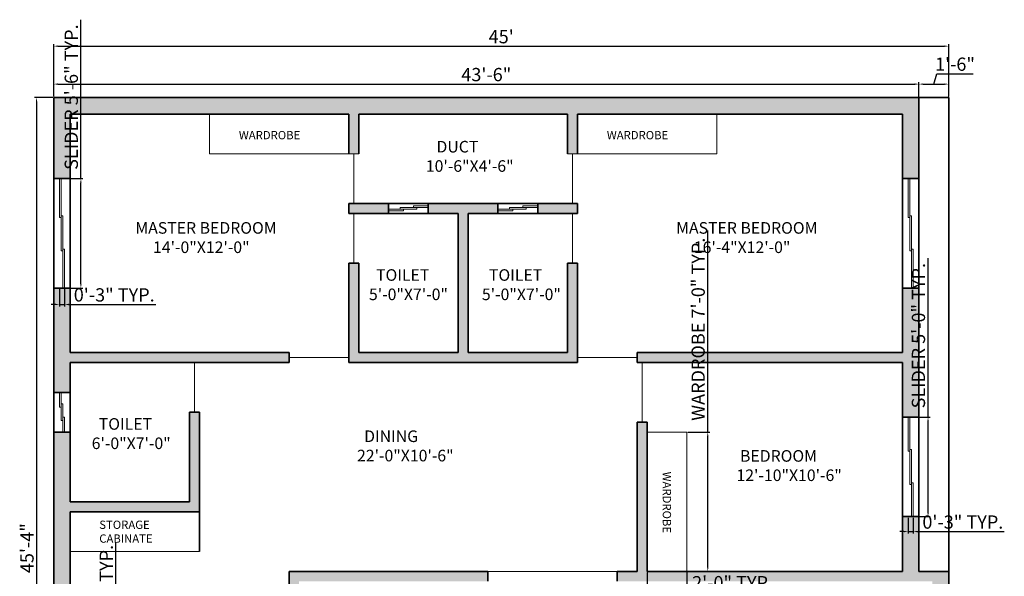
# Model space of a CAD drawing. Units: inches. Extents: x 3491 to 6898, y 1360 to 2019.
# Tile 5 of 9: x 4140 to 4734, y 1683 to 2019. Entities that reach past the tile are written whole.
import ezdxf

# ---------------------------------------------------------------- set-up
doc = ezdxf.new("R2010")
doc.units = ezdxf.units.IN
for name, color, linetype, lineweight in [('A-ANNO-DIMS', 2, 'Continuous', 18), ('A-ANNO-TEXT', 7, 'Continuous', 18), ('A-AREA-IDEN', 7, 'Continuous', 18), ('A-DOOR', 4, 'Continuous', 18), ('A-FLOR-CASE', 8, 'Continuous', 18), ('A-GLAZ', 5, 'Continuous', 18), ('A-WALL', 7, 'Continuous', 35), ('A-WALL-PATT', 8, 'Continuous', 13)]:
    doc.layers.add(name, color=color, linetype=linetype, lineweight=lineweight)
doc.layers.add('A-WALL-OPEN', color=251, linetype='Continuous', lineweight=13, true_color=0x636466)
doc.styles.get("Standard").update_dxf_attribs({"font": 'arial.ttf'})
doc.dimstyles.new('ISO-25', dxfattribs={"dimtxt": 8, "dimasz": 2.5, "dimexe": 1.25, "dimexo": 0.625, "dimtad": 1, "dimdec": 1, "dimlunit": 3, "dimtxsty": 'Standard', "dimcen": 2.5, "dimclrt": 1, "dimadec": 0, "dimazin": 0, "dimtfac": 1, "dimtdec": 1, "dimtmove": 0, "dimatfit": 3, "dimfxl": 1, "dimarcsym": 0})

# ---------------------------------------------------------------- blocks, each defined once
blk = doc.blocks.new('*D15')
at = {"layer": 'A-ANNO-DIMS', "color": 0, "lineweight": -2, "transparency": 16777216}
for p, q in [((4160.3, 1972.99), (4160.3, 1981.69)), ((4162.8, 1980.44), (4679.8, 1980.44)), ((4682.3, 1972.99), (4682.3, 1981.69))]:
    blk.add_line(p, q, dxfattribs=at)
at = {"layer": 'A-ANNO-DIMS', "color": 0, "transparency": 16777216}
for points in [[(4162.8, 1980.85), (4162.8, 1980.02), (4160.3, 1980.44)], [(4679.8, 1980.85), (4679.8, 1980.02), (4682.3, 1980.44)]]:
    blk.add_solid(points, dxfattribs=at)
at = {"layer": 'Defpoints', "color": 0, "transparency": 16777216}
for p in [(4682.3, 1980.44), (4160.3, 1972.37), (4682.3, 1972.37)]:
    blk.add_point(p, dxfattribs=at)
at = {"layer": 'A-ANNO-DIMS', "color": 0, "transparency": 16777216, "insert": (4421.3, 1985.15), "char_height": 8, "attachment_point": 5}
blk.add_mtext('43\'-6"', dxfattribs=at)
blk = doc.blocks.new('*D16')
at = {"layer": 'A-ANNO-DIMS', "color": 0, "lineweight": -2, "transparency": 16777216}
for p, q in [((4691.3, 1980.44), (4693.19, 1986.71)), ((4693.19, 1986.71), (4714.95, 1986.71)), ((4682.3, 1972.99), (4682.3, 1981.69)), ((4684.8, 1980.44), (4697.8, 1980.44)), ((4700.3, 1972.99), (4700.3, 1981.69))]:
    blk.add_line(p, q, dxfattribs=at)
at = {"layer": 'A-ANNO-DIMS', "color": 0, "transparency": 16777216}
for points in [[(4684.8, 1980.85), (4684.8, 1980.02), (4682.3, 1980.44)], [(4697.8, 1980.85), (4697.8, 1980.02), (4700.3, 1980.44)]]:
    blk.add_solid(points, dxfattribs=at)
at = {"layer": 'Defpoints', "color": 0, "transparency": 16777216}
for p in [(4700.3, 1980.44), (4682.3, 1972.37), (4700.3, 1972.37)]:
    blk.add_point(p, dxfattribs=at)
at = {"layer": 'A-ANNO-DIMS', "color": 0, "transparency": 16777216, "insert": (4704.07, 1991.42), "char_height": 8, "attachment_point": 5}
blk.add_mtext('1\'-6"', dxfattribs=at)
blk = doc.blocks.new('*D13')
at = {"layer": 'A-ANNO-DIMS', "color": 0, "lineweight": -2, "transparency": 16777216}
for p, q in [((4160.3, 1972.99), (4160.3, 2004.59)), ((4162.8, 2003.34), (4697.8, 2003.34)), ((4700.3, 1972.99), (4700.3, 2004.59))]:
    blk.add_line(p, q, dxfattribs=at)
at = {"layer": 'A-ANNO-DIMS', "color": 0, "transparency": 16777216}
for points in [[(4162.8, 2003.76), (4162.8, 2002.92), (4160.3, 2003.34)], [(4697.8, 2003.76), (4697.8, 2002.92), (4700.3, 2003.34)]]:
    blk.add_solid(points, dxfattribs=at)
at = {"layer": 'Defpoints', "color": 0, "transparency": 16777216}
for p in [(4700.3, 2003.34), (4160.3, 1972.37), (4700.3, 1972.37)]:
    blk.add_point(p, dxfattribs=at)
at = {"layer": 'A-ANNO-DIMS', "color": 0, "transparency": 16777216, "insert": (4430.3, 2008.03), "char_height": 8, "attachment_point": 5}
blk.add_mtext("45'", dxfattribs=at)
blk = doc.blocks.new('*D17')
at = {"layer": 'A-ANNO-DIMS', "color": 0, "lineweight": -2, "transparency": 16777216}
for p, q in [((4159.68, 1972.37), (4148.67, 1972.37)), ((4149.92, 1969.87), (4149.92, 1430.87)), ((4159.68, 1428.37), (4148.67, 1428.37))]:
    blk.add_line(p, q, dxfattribs=at)
at = {"layer": 'A-ANNO-DIMS', "color": 0, "transparency": 16777216}
for points in [[(4149.51, 1969.87), (4150.34, 1969.87), (4149.92, 1972.37)], [(4149.51, 1430.87), (4150.34, 1430.87), (4149.92, 1428.37)]]:
    blk.add_solid(points, dxfattribs=at)
at = {"layer": 'Defpoints', "color": 0, "transparency": 16777216}
for p in [(4160.3, 1972.37), (4149.92, 1428.37), (4160.3, 1428.37)]:
    blk.add_point(p, dxfattribs=at)
at = {"layer": 'A-ANNO-DIMS', "color": 0, "transparency": 16777216, "insert": (4145.23, 1700.37), "char_height": 8, "attachment_point": 5, "rotation": 90}
blk.add_mtext('45\'-4"', dxfattribs=at)
blk = doc.blocks.new('WIN-SLIDER-24IN')
for p, q in [((0, 1), (17, 1)), ((0, 0), (9, 0)), ((7, 1), (7, 2)), ((7, 2), (24, 2)), ((9, 0), (9, 1)), ((15, 2), (15, 3)), ((15, 3), (24, 3)), ((17, 1), (17, 2))]:
    blk.add_line(p, q)
blk = doc.blocks.new('WIN-SLIDER-66IN')
for p, q in [((0, 42.5), (0, 66)), ((1, 22.5), (1, 66)), ((1, 42.5), (0, 42.5)), ((2, 43.5), (1, 43.5)), ((2, 0), (2, 43.5)), ((2, 22.5), (1, 22.5)), ((3, 23.5), (2, 23.5)), ((3, 0), (3, 23.5))]:
    blk.add_line(p, q)
blk = doc.blocks.new('WIN-SLIDER-60IN')
for p, q in [((0, 39.5), (0, 60)), ((1, 19.5), (1, 60)), ((1, 39.5), (0, 39.5)), ((2, 40.5), (1, 40.5)), ((2, 0), (2, 40.5)), ((2, 19.5), (1, 19.5)), ((3, 20.5), (2, 20.5)), ((3, 0), (3, 20.5))]:
    blk.add_line(p, q)
blk = doc.blocks.new('WARDROBE-84X24')
for q in [(0, 84), (24, 0)]:
    blk.add_line((24, 84), q)
blk = doc.blocks.new('*D114')
at = {"layer": 'A-ANNO-DIMS', "color": 0, "lineweight": -2, "transparency": 16777216}
for p, q in [((4176.7, 1923.37), (4176.7, 2019.32)), ((4167.43, 1923.37), (4177.95, 1923.37)), ((4176.7, 1859.87), (4176.7, 1920.87)), ((4167.43, 1857.37), (4177.95, 1857.37))]:
    blk.add_line(p, q, dxfattribs=at)
at = {"layer": 'A-ANNO-DIMS', "color": 0, "transparency": 16777216}
for points in [[(4176.29, 1920.87), (4177.12, 1920.87), (4176.7, 1923.37)], [(4176.29, 1859.87), (4177.12, 1859.87), (4176.7, 1857.37)]]:
    blk.add_solid(points, dxfattribs=at)
at = {"layer": 'Defpoints', "color": 0, "transparency": 16777216}
for p in [(4166.8, 1923.37), (4176.7, 1923.37), (4166.8, 1857.37)]:
    blk.add_point(p, dxfattribs=at)
at = {"layer": 'A-ANNO-DIMS', "color": 1, "transparency": 16777216, "insert": (4171.94, 1972.59), "char_height": 8, "attachment_point": 5, "rotation": 90}
blk.add_mtext('SLIDER 5\'-6" TYP.', dxfattribs=at)
blk = doc.blocks.new('*D115')
at = {"layer": 'A-ANNO-DIMS', "color": 0, "lineweight": -2, "transparency": 16777216}
for p, q in [((4163.8, 1856.74), (4163.8, 1846.22)), ((4166.8, 1856.74), (4166.8, 1846.22)), ((4161.3, 1847.47), (4158.8, 1847.47)), ((4163.8, 1847.47), (4166.8, 1847.47)), ((4169.3, 1847.47), (4221.82, 1847.47))]:
    blk.add_line(p, q, dxfattribs=at)
at = {"layer": 'A-ANNO-DIMS', "color": 0, "transparency": 16777216}
for points in [[(4161.3, 1847.88), (4161.3, 1847.05), (4163.8, 1847.47)], [(4169.3, 1847.88), (4169.3, 1847.05), (4166.8, 1847.47)]]:
    blk.add_solid(points, dxfattribs=at)
at = {"layer": 'Defpoints', "color": 0, "transparency": 16777216}
for p in [(4163.8, 1857.37), (4166.8, 1857.37), (4166.8, 1847.47)]:
    blk.add_point(p, dxfattribs=at)
at = {"layer": 'A-ANNO-DIMS', "color": 1, "transparency": 16777216, "insert": (4196.81, 1852.18), "char_height": 8, "attachment_point": 5}
blk.add_mtext('0\'-3" TYP.', dxfattribs=at)
blk = doc.blocks.new('*D118')
at = {"layer": 'A-ANNO-DIMS', "color": 0, "lineweight": -2, "transparency": 16777216}
for p, q in [((4687.8, 1779.37), (4687.8, 1875.32)), ((4679.43, 1779.37), (4689.05, 1779.37)), ((4687.8, 1721.87), (4687.8, 1776.87)), ((4679.43, 1719.37), (4689.05, 1719.37))]:
    blk.add_line(p, q, dxfattribs=at)
at = {"layer": 'A-ANNO-DIMS', "color": 0, "transparency": 16777216}
for points in [[(4687.39, 1776.87), (4688.22, 1776.87), (4687.8, 1779.37)], [(4687.39, 1721.87), (4688.22, 1721.87), (4687.8, 1719.37)]]:
    blk.add_solid(points, dxfattribs=at)
at = {"layer": 'Defpoints', "color": 0, "transparency": 16777216}
for p in [(4678.8, 1779.37), (4687.8, 1779.37), (4678.8, 1719.37)]:
    blk.add_point(p, dxfattribs=at)
at = {"layer": 'A-ANNO-DIMS', "color": 1, "transparency": 16777216, "insert": (4683.04, 1828.59), "char_height": 8, "attachment_point": 5, "rotation": 90}
blk.add_mtext('SLIDER 5\'-0" TYP.', dxfattribs=at)
blk = doc.blocks.new('*D119')
at = {"layer": 'A-ANNO-DIMS', "color": 0, "lineweight": -2, "transparency": 16777216}
for p, q in [((4675.8, 1718.74), (4675.8, 1709.12)), ((4678.8, 1718.74), (4678.8, 1709.12)), ((4673.3, 1710.37), (4670.8, 1710.37)), ((4675.8, 1710.37), (4678.8, 1710.37)), ((4681.3, 1710.37), (4733.82, 1710.37))]:
    blk.add_line(p, q, dxfattribs=at)
at = {"layer": 'A-ANNO-DIMS', "color": 0, "transparency": 16777216}
for points in [[(4673.3, 1710.78), (4673.3, 1709.95), (4675.8, 1710.37)], [(4681.3, 1710.78), (4681.3, 1709.95), (4678.8, 1710.37)]]:
    blk.add_solid(points, dxfattribs=at)
at = {"layer": 'Defpoints', "color": 0, "transparency": 16777216}
for p in [(4675.8, 1719.37), (4678.8, 1719.37), (4678.8, 1710.37)]:
    blk.add_point(p, dxfattribs=at)
at = {"layer": 'A-ANNO-DIMS', "color": 1, "transparency": 16777216, "insert": (4708.81, 1715.08), "char_height": 8, "attachment_point": 5}
blk.add_mtext('0\'-3" TYP.', dxfattribs=at)
blk = doc.blocks.new('*D122')
at = {"layer": 'A-ANNO-DIMS', "color": 0, "lineweight": -2, "transparency": 16777216}
for p, q in [((4554.9, 1770.37), (4554.9, 1892.13)), ((4542.93, 1770.37), (4556.15, 1770.37)), ((4554.9, 1688.87), (4554.9, 1767.87)), ((4542.93, 1686.37), (4556.15, 1686.37))]:
    blk.add_line(p, q, dxfattribs=at)
at = {"layer": 'A-ANNO-DIMS', "color": 0, "transparency": 16777216}
for points in [[(4554.49, 1767.87), (4555.32, 1767.87), (4554.9, 1770.37)], [(4554.49, 1688.87), (4555.32, 1688.87), (4554.9, 1686.37)]]:
    blk.add_solid(points, dxfattribs=at)
at = {"layer": 'Defpoints', "color": 0, "transparency": 16777216}
for p in [(4542.3, 1770.37), (4554.9, 1770.37), (4542.3, 1686.37)]:
    blk.add_point(p, dxfattribs=at)
at = {"layer": 'A-ANNO-DIMS', "color": 1, "transparency": 16777216, "insert": (4550.14, 1832.5), "char_height": 8, "attachment_point": 5, "rotation": 90}
blk.add_mtext('WARDROBE 7\'-0" TYP.', dxfattribs=at)
blk = doc.blocks.new('*D123')
at = {"layer": 'A-ANNO-DIMS', "color": 0, "lineweight": -2, "transparency": 16777216}
for p, q in [((4518.3, 1685.74), (4518.3, 1672.52)), ((4542.3, 1685.74), (4542.3, 1672.52)), ((4520.8, 1673.77), (4539.8, 1673.77)), ((4542.3, 1673.77), (4594.96, 1673.77))]:
    blk.add_line(p, q, dxfattribs=at)
at = {"layer": 'A-ANNO-DIMS', "color": 0, "transparency": 16777216}
for points in [[(4520.8, 1674.18), (4520.8, 1673.35), (4518.3, 1673.77)], [(4539.8, 1674.18), (4539.8, 1673.35), (4542.3, 1673.77)]]:
    blk.add_solid(points, dxfattribs=at)
at = {"layer": 'Defpoints', "color": 0, "transparency": 16777216}
for p in [(4518.3, 1686.37), (4542.3, 1686.37), (4542.3, 1673.77)]:
    blk.add_point(p, dxfattribs=at)
at = {"layer": 'A-ANNO-DIMS', "color": 1, "transparency": 16777216, "insert": (4569.88, 1678.48), "char_height": 8, "attachment_point": 5}
blk.add_mtext('2\'-0" TYP.', dxfattribs=at)
blk = doc.blocks.new('*D126')
at = {"layer": 'A-ANNO-DIMS', "color": 0, "lineweight": -2, "transparency": 16777216}
for p, q in [((4197.86, 1622.3), (4197.86, 1703.97)), ((4193.08, 1622.3), (4199.11, 1622.3)), ((4197.86, 1588.8), (4197.86, 1619.8)), ((4193.08, 1586.3), (4199.11, 1586.3))]:
    blk.add_line(p, q, dxfattribs=at)
at = {"layer": 'A-ANNO-DIMS', "color": 0, "transparency": 16777216}
for points in [[(4197.44, 1619.8), (4198.27, 1619.8), (4197.86, 1622.3)], [(4197.44, 1588.8), (4198.27, 1588.8), (4197.86, 1586.3)]]:
    blk.add_solid(points, dxfattribs=at)
at = {"layer": 'Defpoints', "color": 0, "transparency": 16777216}
for p in [(4192.46, 1622.3), (4197.86, 1622.3), (4192.46, 1586.3)]:
    blk.add_point(p, dxfattribs=at)
at = {"layer": 'A-ANNO-DIMS', "color": 1, "transparency": 16777216, "insert": (4193.09, 1664.39), "char_height": 8, "attachment_point": 5, "rotation": 90}
blk.add_mtext('SINK 3\'-0" TYP.', dxfattribs=at)

msp = doc.modelspace()

# ---------------------------------------------------------------- hatches: boundary and pattern name
at = {"layer": 'A-WALL-PATT'}
h = msp.add_hatch(color=256, dxfattribs=at)
h.dxf.hatch_style = 1
h.paths.add_polyline_path([(4484.3, 1532.37), (4476.3, 1532.37), (4452.32, 1532.37), (4452.32, 1522.37), (4484.3, 1522.37)])
h.paths.add_polyline_path([(4534.3, 1556.37), (4524.3, 1556.37), (4524.3, 1532.37), (4520.3, 1532.37), (4520.3, 1522.37), (4524.3, 1522.37), (4524.3, 1486.37), (4561.28, 1486.37), (4561.28, 1496.37), (4534.3, 1496.37)], flags=17)
h.paths.add_polyline_path([(4404.32, 1532.37), (4356.3, 1532.37), (4356.3, 1522.37), (4404.32, 1522.37)], flags=17)
h.paths.add_polyline_path([(4648.3, 1496.37), (4621.28, 1496.37), (4621.28, 1486.37), (4648.3, 1486.37)], flags=17)
h.paths.add_polyline_path([(4700.3, 1686.37), (4682.3, 1686.37), (4682.3, 1719.37), (4672.3, 1719.37), (4672.3, 1686.37), (4518.3, 1686.37), (4518.3, 1776.37), (4512.3, 1776.37), (4512.3, 1686.37), (4500.3, 1686.37), (4500.3, 1680.37), (4690.3, 1680.37), (4690.3, 1496.37), (4678.3, 1496.37), (4678.3, 1486.37), (4700.3, 1486.37)])
h.paths.add_polyline_path([(4422.3, 1686.37), (4302.3, 1686.37), (4302.3, 1532.37), (4284.33, 1532.37), (4284.33, 1522.37), (4314.3, 1522.37), (4314.3, 1532.37), (4308.3, 1532.37), (4308.3, 1680.37), (4422.3, 1680.37)])
h.paths.add_polyline_path([(4170.3, 1722.37), (4248.3, 1722.37), (4248.3, 1782.37), (4242.3, 1782.37), (4242.3, 1728.37), (4170.3, 1728.37), (4170.3, 1770.37), (4160.3, 1770.37), (4160.3, 1628.4), (4170.3, 1628.4)])
h.paths.add_polyline_path([(4170.3, 1580.4), (4160.3, 1580.4), (4160.3, 1428.37), (4302.3, 1428.37), (4302.3, 1438.37), (4170.3, 1438.37), (4170.3, 1522.37), (4236.33, 1522.37), (4236.33, 1532.37), (4170.3, 1532.37)])
h.paths.add_polyline_path([(4368.3, 1486.37), (4362.3, 1486.37), (4362.3, 1428.37), (4368.3, 1428.37)])
h.paths.add_polyline_path([(4682.3, 1857.37), (4672.3, 1857.37), (4672.3, 1818.37), (4512.3, 1818.37), (4512.3, 1812.37), (4672.3, 1812.37), (4672.3, 1779.37), (4682.3, 1779.37)])
h.paths.add_polyline_path([(4476.3, 1872.37), (4470.3, 1872.37), (4470.3, 1818.37), (4410.3, 1818.37), (4410.3, 1902.37), (4428.3, 1902.37), (4428.3, 1908.37), (4386.3, 1908.37), (4386.3, 1902.37), (4404.3, 1902.37), (4404.3, 1818.37), (4344.3, 1818.37), (4344.3, 1872.37), (4338.3, 1872.37), (4338.3, 1812.37), (4476.3, 1812.37)])
h.paths.add_polyline_path([(4170.3, 1857.37), (4160.3, 1857.37), (4160.3, 1794.37), (4170.3, 1794.37), (4170.3, 1812.37), (4302.3, 1812.37), (4302.3, 1818.37), (4170.3, 1818.37)])
h.paths.add_polyline_path([(4170.3, 1962.37), (4338.3, 1962.37), (4338.3, 1938.37), (4344.3, 1938.37), (4344.3, 1962.37), (4470.3, 1962.37), (4470.3, 1938.37), (4476.3, 1938.37), (4476.3, 1962.37), (4672.3, 1962.37), (4672.3, 1923.37), (4682.3, 1923.37), (4682.3, 1972.37), (4160.3, 1972.37), (4160.3, 1923.37), (4170.3, 1923.37)])
h.paths.add_polyline_path([(4476.3, 1908.37), (4452.3, 1908.37), (4452.3, 1902.37), (4476.3, 1902.37)], flags=17)
h.paths.add_polyline_path([(4362.3, 1908.37), (4338.3, 1908.37), (4338.3, 1902.37), (4362.3, 1902.37)], flags=17)

# ---------------------------------------------------------------- linework, layer by layer
at = {"layer": 'A-DOOR'}
for p, q in [((4341.3, 1938.37), (4341.3, 1908.37)), ((4473.3, 1938.37), (4473.3, 1908.37)), ((4341.3, 1872.37), (4341.3, 1902.37)), ((4473.3, 1872.37), (4473.3, 1902.37)), ((4245.3, 1782.37), (4245.3, 1812.37)), ((4302.3, 1815.37), (4338.3, 1815.37)), ((4512.3, 1815.37), (4476.3, 1815.37)), ((4515.3, 1776.37), (4515.3, 1812.37))]:
    msp.add_line(p, q, dxfattribs=at)
at = {"layer": 'A-FLOR-CASE'}
for p, q in [((4254.3, 1962.37), (4254.3, 1938.37)), ((4560.3, 1962.37), (4560.3, 1938.37)), ((4344.3, 1938.37), (4254.3, 1938.37)), ((4560.3, 1938.37), (4470.3, 1938.37)), ((4248.3, 1698.37), (4170.3, 1698.37))]:
    msp.add_line(p, q, dxfattribs=at)
at = {"layer": 'A-WALL'}
for p, q in [((4700.3, 1972.37), (4160.3, 1972.37)), ((4160.3, 1972.37), (4160.3, 1428.37)), ((4682.3, 1972.37), (4682.3, 1686.37)), ((4700.3, 1428.37), (4700.3, 1972.37)), ((4338.3, 1962.37), (4170.3, 1962.37)), ((4170.3, 1962.37), (4170.3, 1818.37)), ((4338.3, 1962.37), (4338.3, 1938.37)), ((4470.3, 1962.37), (4344.3, 1962.37)), ((4344.3, 1962.37), (4344.3, 1938.37)), ((4470.3, 1962.37), (4470.3, 1938.37)), ((4672.3, 1962.37), (4476.3, 1962.37)), ((4476.3, 1962.37), (4476.3, 1938.37)), ((4672.3, 1962.37), (4672.3, 1818.37)), ((4170.3, 1923.37), (4160.3, 1923.37)), ((4682.3, 1923.37), (4672.3, 1923.37)), ((4338.3, 1908.37), (4338.3, 1902.37)), ((4476.3, 1908.37), (4338.3, 1908.37)), ((4362.3, 1908.37), (4362.3, 1902.37)), ((4386.3, 1908.37), (4386.3, 1902.37)), ((4428.3, 1908.37), (4428.3, 1902.37)), ((4452.3, 1908.37), (4452.3, 1902.37)), ((4476.3, 1908.37), (4476.3, 1902.37)), ((4404.3, 1902.37), (4338.3, 1902.37)), ((4404.3, 1902.37), (4404.3, 1818.37)), ((4410.3, 1902.37), (4410.3, 1818.37)), ((4476.3, 1902.37), (4410.3, 1902.37)), ((4338.3, 1872.37), (4338.3, 1812.37)), ((4344.3, 1872.37), (4338.3, 1872.37)), ((4344.3, 1872.37), (4344.3, 1818.37)), ((4470.3, 1872.37), (4470.3, 1818.37)), ((4476.3, 1872.37), (4470.3, 1872.37)), ((4476.3, 1872.37), (4476.3, 1812.37)), ((4170.3, 1857.37), (4160.3, 1857.37)), ((4682.3, 1857.37), (4672.3, 1857.37)), ((4302.3, 1818.37), (4170.3, 1818.37)), ((4302.3, 1818.37), (4302.3, 1812.37)), ((4404.3, 1818.37), (4344.3, 1818.37)), ((4470.3, 1818.37), (4410.3, 1818.37)), ((4672.3, 1818.37), (4512.3, 1818.37)), ((4512.3, 1818.37), (4512.3, 1812.37)), ((4302.3, 1812.37), (4170.3, 1812.37)), ((4170.3, 1812.37), (4170.3, 1728.37)), ((4476.3, 1812.37), (4338.3, 1812.37)), ((4672.3, 1812.37), (4512.3, 1812.37)), ((4672.3, 1812.37), (4672.3, 1686.37)), ((4170.3, 1794.37), (4160.3, 1794.37)), ((4248.3, 1782.37), (4242.3, 1782.37)), ((4242.3, 1782.37), (4242.3, 1728.37)), ((4248.3, 1782.37), (4248.3, 1698.37)), ((4518.3, 1776.37), (4512.3, 1776.37)), ((4512.3, 1776.37), (4512.3, 1686.37)), ((4518.3, 1776.37), (4518.3, 1686.37)), ((4682.3, 1779.37), (4672.3, 1779.37)), ((4170.3, 1770.37), (4160.3, 1770.37)), ((4242.3, 1728.37), (4170.3, 1728.37)), ((4248.3, 1722.37), (4170.3, 1722.37)), ((4170.3, 1722.37), (4170.3, 1532.37)), ((4682.3, 1719.37), (4672.3, 1719.37)), ((4422.3, 1686.37), (4302.3, 1686.37)), ((4302.3, 1686.37), (4302.3, 1532.37)), ((4422.3, 1686.37), (4422.3, 1680.37)), ((4512.3, 1686.37), (4500.3, 1686.37)), ((4500.3, 1686.37), (4500.3, 1680.37)), ((4672.3, 1686.37), (4518.3, 1686.37)), ((4700.3, 1686.37), (4682.3, 1686.37))]:
    msp.add_line(p, q, dxfattribs=at)
at = {"layer": 'A-WALL-OPEN'}
msp.add_line((4500.3, 1686.37), (4422.3, 1686.37), dxfattribs=at)

# ---------------------------------------------------------------- block references
at = {"layer": 'A-FLOR-CASE'}
msp.add_blockref('WARDROBE-84X24', (4518.3, 1686.37), dxfattribs=at)
at = {"layer": 'A-GLAZ'}
for name, p in [('WIN-SLIDER-66IN', (4163.8, 1857.37)), ('WIN-SLIDER-66IN', (4675.8, 1857.37)), ('WIN-SLIDER-24IN', (4362.3, 1903.87)), ('WIN-SLIDER-24IN', (4428.3, 1903.87)), ('WIN-SLIDER-60IN', (4675.8, 1719.37))]:
    msp.add_blockref(name, p, dxfattribs=at)
at = {"layer": 'A-GLAZ', "rotation": 270}
msp.add_blockref('WIN-SLIDER-24IN', (4163.8, 1794.37), dxfattribs=at)

# ---------------------------------------------------------------- texts
at = {"layer": 'A-ANNO-TEXT', "char_height": 5, "attachment_point": 1}
for s, insert in [('WARDROBE', (4272.01, 1952.13)), ('WARDROBE', (4494.01, 1952.13)), ('STORAGE\\PCABINATE', (4187.79, 1716.98))]:
    msp.add_mtext_dynamic_manual_height_columns(s, width=86.9528, gutter_width=12.5, heights=[0], dxfattribs=dict(at, insert=insert))
at = {"layer": 'A-ANNO-TEXT', "insert": (4532.75, 1746.53), "char_height": 5, "attachment_point": 1, "rotation": 270}
msp.add_mtext_dynamic_manual_height_columns('WARDROBE', width=86.9528, gutter_width=12.5, heights=[0], dxfattribs=at)
at = {"layer": 'A-AREA-IDEN', "char_height": 7, "attachment_point": 1}
for s, heights, insert in [('   DUCT\\P10\'-6"X4\'-6"', [0], (4384.81, 1946.16)), ('MASTER BEDROOM\\P     14\'-0"X12\'-0"', [0], (4209.54, 1897.15)), ('MASTER BEDROOM\\P     16\'-4"X12\'-0"', [0], (4535.83, 1897.15)), ('  TOILET\\P5\'-0"X7\'-0"', [0], (4350.5, 1868.72)), ('  TOILET\\P5\'-0"X7\'-0"', [0], (4418.64, 1868.72)), ('  TOILET\\P6\'-0"X7\'-0"', [0], (4183.22, 1778.82)), ('  DINING\\P22\'-0"X10\'-6"', [18.93], (4343.31, 1771.4)), (' BEDROOM\\P12\'-10"X10\'-6"', [0], (4572.22, 1759.53))]:
    msp.add_mtext_dynamic_manual_height_columns(s, width=121.6144, gutter_width=12.5, heights=heights, dxfattribs=dict(at, insert=insert))

# ---------------------------------------------------------------- dimensions: what is measured, and where the dimension line sits
at = {"layer": 'A-ANNO-DIMS'}
for base, p1, p2, text, picture, middle in [((4176.7, 1923.37), (4166.8, 1857.37), (4166.8, 1923.37), 'SLIDER <> TYP.', '*D114', (4171.94, 1972.59)), ((4554.9, 1770.37), (4542.3, 1686.37), (4542.3, 1770.37), 'WARDROBE <> TYP.', '*D122', (4550.14, 1832.5)), ((4687.8, 1779.37), (4678.8, 1719.37), (4678.8, 1779.37), 'SLIDER <> TYP.', '*D118', (4683.04, 1828.59)), ((4197.86, 1622.3), (4192.46, 1586.3), (4192.46, 1622.3), 'SINK <> TYP.', '*D126', (4193.09, 1664.39))]:
    dim = msp.add_linear_dim(base=base, p1=p1, p2=p2, angle=90, text=text, dimstyle='ISO-25', override={"dimdec": 1, "dimlfac": 1, "dimrnd": 0, "dimzin": 1, "dimdsep": 46, "dimlunit": 4, "dimfrac": 2}, dxfattribs=at)
    dim.commit()
    dim.dimension.update_dxf_attribs({"geometry": picture, "text_midpoint": middle})
for base, p1, p2, override, picture, middle in [((4700.3, 2003.34), (4160.3, 1972.37), (4700.3, 1972.37), {"dimclrd": 0, "dimclre": 0, "dimclrt": 0}, '*D13', (4430.3, 2008.03)), ((4700.3, 1980.44), (4682.3, 1972.37), (4700.3, 1972.37), {"dimclrd": 0, "dimclre": 0, "dimclrt": 0, "dimtmove": 1}, '*D16', (4693.81, 1991.42)), ((4682.3, 1980.44), (4160.3, 1972.37), (4682.3, 1972.37), {"dimclrd": 0, "dimclre": 0, "dimclrt": 0}, '*D15', (4421.3, 1985.15))]:
    dim = msp.add_linear_dim(base=base, p1=p1, p2=p2, dimstyle='ISO-25', override=override, dxfattribs=at)
    dim.commit()
    dim.dimension.update_dxf_attribs({"geometry": picture, "text_midpoint": middle})
dim = msp.add_linear_dim(base=(4149.92, 1428.37), p1=(4160.3, 1972.37), p2=(4160.3, 1428.37), angle=90, dimstyle='ISO-25', override={"dimclrd": 0, "dimclre": 0, "dimclrt": 0}, dxfattribs=at)
dim.commit()
dim.dimension.update_dxf_attribs({"geometry": '*D17', "text_midpoint": (4145.23, 1700.37)})
for base, p1, p2, picture, middle in [((4166.8, 1847.47), (4163.8, 1857.37), (4166.8, 1857.37), '*D115', (4196.81, 1852.18)), ((4678.8, 1710.37), (4675.8, 1719.37), (4678.8, 1719.37), '*D119', (4708.81, 1715.08)), ((4542.3, 1673.77), (4518.3, 1686.37), (4542.3, 1686.37), '*D123', (4569.88, 1678.48))]:
    dim = msp.add_linear_dim(base=base, p1=p1, p2=p2, text='<> TYP.', dimstyle='ISO-25', override={"dimdec": 1, "dimlfac": 1, "dimrnd": 0, "dimzin": 1, "dimdsep": 46, "dimlunit": 4, "dimfrac": 2}, dxfattribs=at)
    dim.commit()
    dim.dimension.update_dxf_attribs({"geometry": picture, "text_midpoint": middle})

doc.saveas('drawing.dxf')
